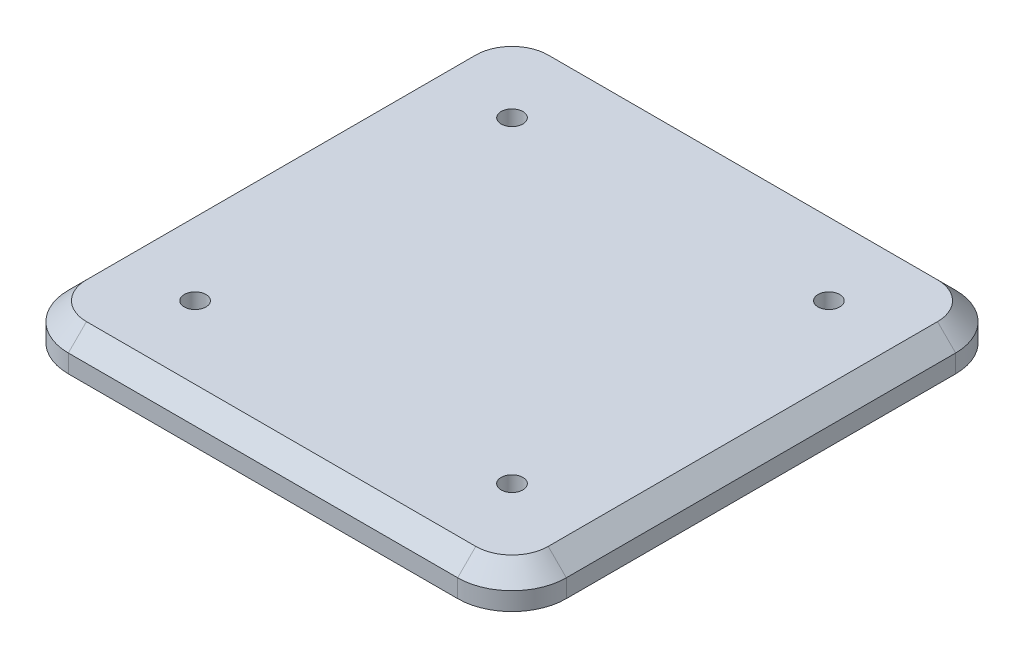
from build123d import *

# Parameters (mm, degrees)
BASE_PLATE_PROFILE_275X275_W       = 275
BASE_PLATE_PROFILE_275X275_H       = 275
BASE_PLATE_275X275X20_DEPTH        = 20
CORNER_FILLETS_R30_R               = 30
EDGE_CHAMFER_10X45_SIZE            = 10
DOWEL_HOLES_12_ON_175_SQUARE_D     = 12
DOWEL_HOLES_12_ON_175_SQUARE_DEPTH = 10
DOWEL_HOLES_12_ON_175_SQUARE_TIP   = 3.605163714
DOWEL_HOLES_12_ON_225_SQUARE_D     = 12
DOWEL_HOLES_12_ON_225_SQUARE_DEPTH = 10
DOWEL_HOLES_12_ON_225_SQUARE_TIP   = 3.605163714


with BuildPart() as part:
    # Base Plate Profile 275x275 → Base Plate 275x275x20 (new body)
    with BuildSketch(Plane(origin=(0, 0, 0), x_dir=(1, 0, 0), z_dir=(0, 1, 0))):
        Rectangle(BASE_PLATE_PROFILE_275X275_W, BASE_PLATE_PROFILE_275X275_H)
    extrude(amount=BASE_PLATE_275X275X20_DEPTH)

    # Corner Fillets R30
    corner_fillets_r30_edges = [part.edges().sort_by_distance(p)[0] for p in [
        (-137.5, 10, 137.5),
        (-137.5, 10, -137.5),
        (137.5, 10, -137.5),
        (137.5, 10, 137.5),
    ]]
    fillet(corner_fillets_r30_edges, radius=CORNER_FILLETS_R30_R)

    # Edge Chamfer 10x45
    edge_chamfer_10x45_edges = [part.edges().sort_by_distance(p)[0] for p in [
        (0, 20, -137.5),
        (137.5, 20, 0),
        (0, 20, 137.5),
        (-137.5, 20, 0),
        (-128.713203436, 20, 128.713203436),
        (128.713203436, 20, 128.713203436),
        (-128.713203436, 20, -128.713203436),
        (128.713203436, 20, -128.713203436),
    ]]
    chamfer(edge_chamfer_10x45_edges, length=EDGE_CHAMFER_10X45_SIZE)

    # Dowel Holes Ø12 on 175 Square
    with Locations(Plane(origin=(-87.5, 20, -87.5), x_dir=(0, 0, 1), z_dir=(0, 1, 0))):
        with Locations((0, 0), (0, 175), (175, 175), (175, 0)):
            Hole(DOWEL_HOLES_12_ON_175_SQUARE_D / 2, depth=DOWEL_HOLES_12_ON_175_SQUARE_DEPTH)
            with Locations((0, 0, -(DOWEL_HOLES_12_ON_175_SQUARE_DEPTH + DOWEL_HOLES_12_ON_175_SQUARE_TIP / 2))):  # 118° drill point
                Cone(0, DOWEL_HOLES_12_ON_175_SQUARE_D / 2, DOWEL_HOLES_12_ON_175_SQUARE_TIP, mode=Mode.SUBTRACT)

    # Dowel Holes Ø12 on 225 Square
    with Locations(Plane(origin=(-112.5, 0, 112.5), x_dir=(0, 0, -1), z_dir=(0, -1, 0))):
        with Locations((0, 0), (0, 225), (225, 225), (225, 0)):
            Hole(DOWEL_HOLES_12_ON_225_SQUARE_D / 2, depth=DOWEL_HOLES_12_ON_225_SQUARE_DEPTH)
            with Locations((0, 0, -(DOWEL_HOLES_12_ON_225_SQUARE_DEPTH + DOWEL_HOLES_12_ON_225_SQUARE_TIP / 2))):  # 118° drill point
                Cone(0, DOWEL_HOLES_12_ON_225_SQUARE_D / 2, DOWEL_HOLES_12_ON_225_SQUARE_TIP, mode=Mode.SUBTRACT)


solid = part.part
